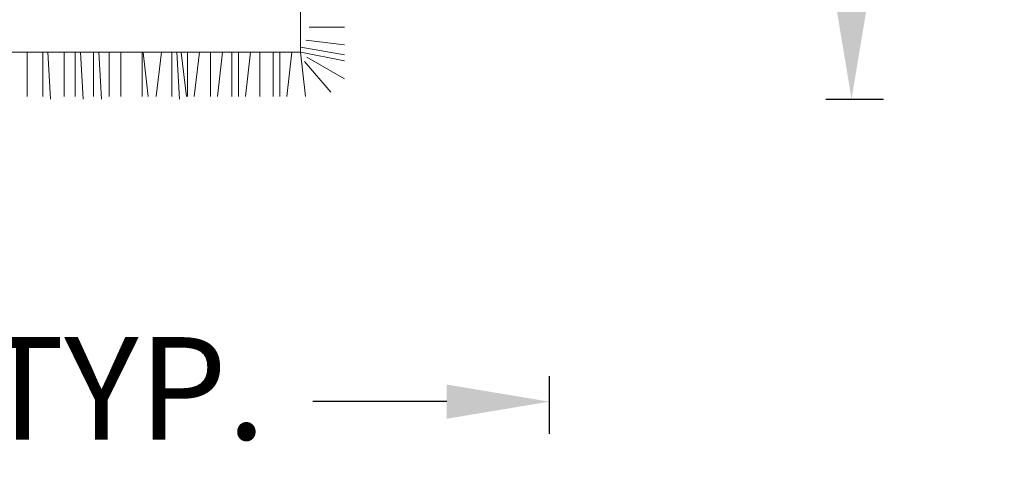
# Model space of a CAD drawing. Units: inches. Extents: x -638 to 186, y -762 to 59.
# Tile 24 of 31: x -66 to -27, y -126 to -108. Entities that reach past the tile are written whole.
import ezdxf

# ---------------------------------------------------------------- set-up
doc = ezdxf.new("R2010")
doc.units = ezdxf.units.IN
doc.layers.add('A-ANNO-DIMS', color=2, linetype='Continuous', lineweight=18)
doc.layers.add('furn', color=8, linetype='Continuous', lineweight=13)
doc.styles.get("Standard").update_dxf_attribs({"font": 'arial.ttf'})
doc.dimstyles.new('ISO-25', dxfattribs={"dimtxt": 4, "dimasz": 4, "dimexe": 1.25, "dimexo": 0.625, "dimtad": 0, "dimlunit": 4, "dimtxsty": 'Standard', "dimcen": 2.5, "dimclrt": 256, "dimadec": 0, "dimazin": 0, "dimtfac": 1, "dimtmove": 0, "dimatfit": 3, "dimfxl": 1, "dimfxlon": 1, "dimarcsym": 0})

# ---------------------------------------------------------------- blocks, each defined once
blk = doc.blocks.new('BED-DOUBLE-WITH-NIGHTSTANDS')
for p, q in [((68.982, 31.914), (68.982, 1.829)), ((69.331, 2.81), (70.707, 2.81)), ((68.996, 2.022), (70.707, 1.732)), ((69.195, 2.295), (70.71, 2.115)), ((68.982, 1.829), (38.435, 1.829)), ((58.312, 1.829), (58.312, 0.102)), ((58.923, 1.829), (58.923, 0.102)), ((59.126, 1.829), (59.228, 0)), ((59.755, 1.815), (59.755, 0.105)), ((60.193, 1.829), (60.193, 0.102)), ((60.397, 1.829), (60.499, 0)), ((60.906, 1.829), (60.906, 0.102)), ((61.11, 1.829), (61.212, 0)), ((61.517, 1.829), (61.517, 0.102)), ((61.977, 1.829), (61.977, 0.102)), ((62.81, 1.815), (62.81, 0.105)), ((62.841, 1.815), (63.044, 0.102)), ((63.554, 1.829), (63.35, 0.102)), ((63.961, 1.829), (63.961, 0.102)), ((64.165, 1.829), (64.266, 0)), ((64.327, 1.815), (64.531, 0.102)), ((64.572, 1.829), (64.572, 0.102)), ((65.04, 1.829), (64.836, 0.102)), ((65.476, 1.829), (65.476, 0.102)), ((65.944, 1.829), (65.741, 0.102)), ((66.309, 1.815), (66.309, 0.105)), ((66.573, 1.829), (66.573, 0.102)), ((67.041, 1.829), (66.838, 0.102)), ((67.406, 1.815), (67.406, 0.105)), ((67.922, 1.815), (67.922, 0.105)), ((68.186, 1.829), (68.186, 0.102)), ((68.654, 1.829), (68.45, 0.102)), ((68.982, 1.829), (69.186, 0.102)), ((68.996, 1.829), (70.707, 1.486)), ((69.232, 1.631), (70.71, 0.792)), ((69.142, 1.47), (70.169, 0.275))]:
    blk.add_line(p, q)
blk = doc.blocks.new('*D27')
at = {"layer": 'A-ANNO-DIMS', "color": 0, "lineweight": -2, "transparency": 16777216}
for p, q in [((-123.625, -121.818), (-123.625, -124.068)), ((-44.925, -121.818), (-44.925, -124.068)), ((-119.625, -122.818), (-114.394, -122.818)), ((-48.925, -122.818), (-54.156, -122.818))]:
    blk.add_line(p, q, dxfattribs=at)
at = {"layer": 'A-ANNO-DIMS', "color": 0, "lineweight": 30, "transparency": 16777216}
for points in [[(-119.625, -122.151), (-119.625, -123.485), (-123.625, -122.818)], [(-48.925, -122.151), (-48.925, -123.485), (-44.925, -122.818)]]:
    blk.add_solid(points, dxfattribs=at)
at = {"layer": 'Defpoints', "color": 0, "lineweight": 30, "transparency": 16777216}
for p in [(-123.625, -111.013), (-44.925, -111.013), (-44.925, -122.818)]:
    blk.add_point(p, dxfattribs=at)
at = {"layer": 'A-ANNO-DIMS', "transparency": 16777216, "insert": (-84.275, -122.818), "char_height": 4, "attachment_point": 5}
blk.add_mtext('BED SET 6\'-6 1/2" TYP.', dxfattribs=at)
blk = doc.blocks.new('*D28')
at = {"layer": 'A-ANNO-DIMS', "color": 0, "lineweight": -2, "transparency": 16777216}
for p, q in [((-34.121, -51.062), (-31.871, -51.062)), ((-33.121, -55.062), (-33.121, -68.221)), ((-33.121, -107.013), (-33.121, -93.853)), ((-34.121, -111.013), (-31.871, -111.013))]:
    blk.add_line(p, q, dxfattribs=at)
at = {"layer": 'A-ANNO-DIMS', "color": 0, "lineweight": 30, "transparency": 16777216}
for points in [[(-33.787, -55.062), (-32.454, -55.062), (-33.121, -51.062)], [(-33.787, -107.013), (-32.454, -107.013), (-33.121, -111.013)]]:
    blk.add_solid(points, dxfattribs=at)
at = {"layer": 'Defpoints', "color": 0, "lineweight": 30, "transparency": 16777216}
for p in [(-44.925, -51.062), (-33.121, -51.062), (-44.925, -111.013)]:
    blk.add_point(p, dxfattribs=at)
at = {"layer": 'A-ANNO-DIMS', "transparency": 16777216, "insert": (-33.121, -81.037), "char_height": 4, "attachment_point": 5, "rotation": 90}
blk.add_mtext('5\'-0" TYP.', dxfattribs=at)

msp = doc.modelspace()

# ---------------------------------------------------------------- block references
at = {"layer": 'furn'}
msp.add_blockref('BED-DOUBLE-WITH-NIGHTSTANDS', (-123.625, -111.013), dxfattribs=at)

# ---------------------------------------------------------------- dimensions: what is measured, and where the dimension line sits
at = {"layer": 'A-ANNO-DIMS'}
dim = msp.add_linear_dim(base=(-33.121, -51.062), p1=(-44.925, -111.013), p2=(-44.925, -51.062), angle=90, text='<> TYP.', dimstyle='ISO-25', override={"dimdec": 1, "dimlfac": 1, "dimrnd": 0, "dimzin": 1, "dimdsep": 46, "dimlunit": 4, "dimfrac": 2}, dxfattribs=at)
dim.commit()
dim.dimension.update_dxf_attribs({"geometry": '*D28', "text_midpoint": (-33.121, -81.037)})
dim = msp.add_linear_dim(base=(-44.925, -122.818), p1=(-123.625, -111.013), p2=(-44.925, -111.013), text='BED SET <> TYP.', dimstyle='ISO-25', override={"dimdec": 1, "dimlfac": 1, "dimrnd": 0, "dimzin": 1, "dimdsep": 46, "dimlunit": 4, "dimfrac": 2}, dxfattribs=at)
dim.commit()
dim.dimension.update_dxf_attribs({"geometry": '*D27', "text_midpoint": (-84.275, -122.818)})

doc.saveas('drawing.dxf')
